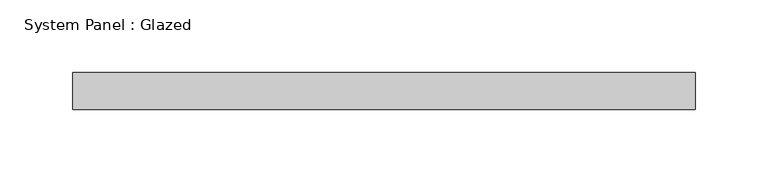
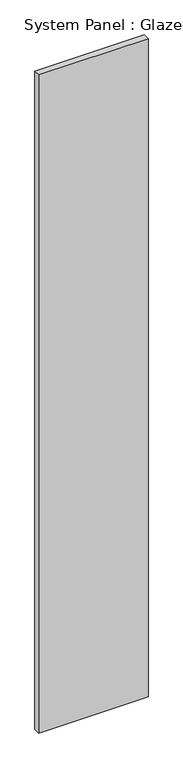
"""IFC4 building model written with IfcOpenShell, lengths in millimetres: plate geometry, System Panel : Glazed."""

from ifc_helpers import new_model, si_unit, origin, origin_with_axes, place, context, project, spatial, polyline, outline, extrude, source, transform, mapped, element, save


def system_panel_glazed_76cbe525(model_context):
    return source(origin(), model_context, "Body", "SweptSolid", [
        extrude(outline(polyline([(213.7833333, 19.05), (-213.7833333, 19.05), (-213.7833333, 44.45), (213.7833333, 44.45), (213.7833333, 19.05)])), origin_with_axes(), (0.0, 0.0, 1.0), 2719.788773),
    ])


if __name__ == "__main__":
    model = new_model("IFC4")
    model_context = context("Model", 3, world=origin())
    ifc_project = project(units=[si_unit("LENGTHUNIT", "METRE", prefix="MILLI")], contexts=[model_context])
    site = spatial("IfcSite", under=ifc_project)
    building = spatial("IfcBuilding", under=site)
    placement = place(None, origin())
    system_panel_glazed_shape = system_panel_glazed_76cbe525(model_context)
    element("IfcPlate", 1, ObjectType="System Panel : Glazed", at=placement, inside=building, context=model_context, shape_type="MappedRepresentation", body=[
        mapped(system_panel_glazed_shape, transform((0.0, 0.0, 0.0), x_axis=(1.0, 0.0, 0.0), y_axis=(0.0, 1.0, 0.0), z_axis=(0.0, 0.0, 1.0))),
    ])
    save(model, "model.ifc")

# Revit data of these elements
# Type "System Panel : Glazed"
#   Construction Type Id = "GSP4R"
#   Analytic Construction = "1/8 in Pilkington single glazing"
#   Visual Light Transmittance = 0.9
#   Solar Heat Gain Coefficient = 0.86
#   Heat Transfer Coefficient (U) = 1.18115 BTU/(h·ft²·°F)
# Element 1 (IfcPlate, "System Panel : Glazed")
#   Materials on its faces: "Glass"
# Materials
#   "Glass": class "Glass", colour RGB 0 128 192, transparency 0.75, Description = "Soda Lime Glass", Cost = 0
